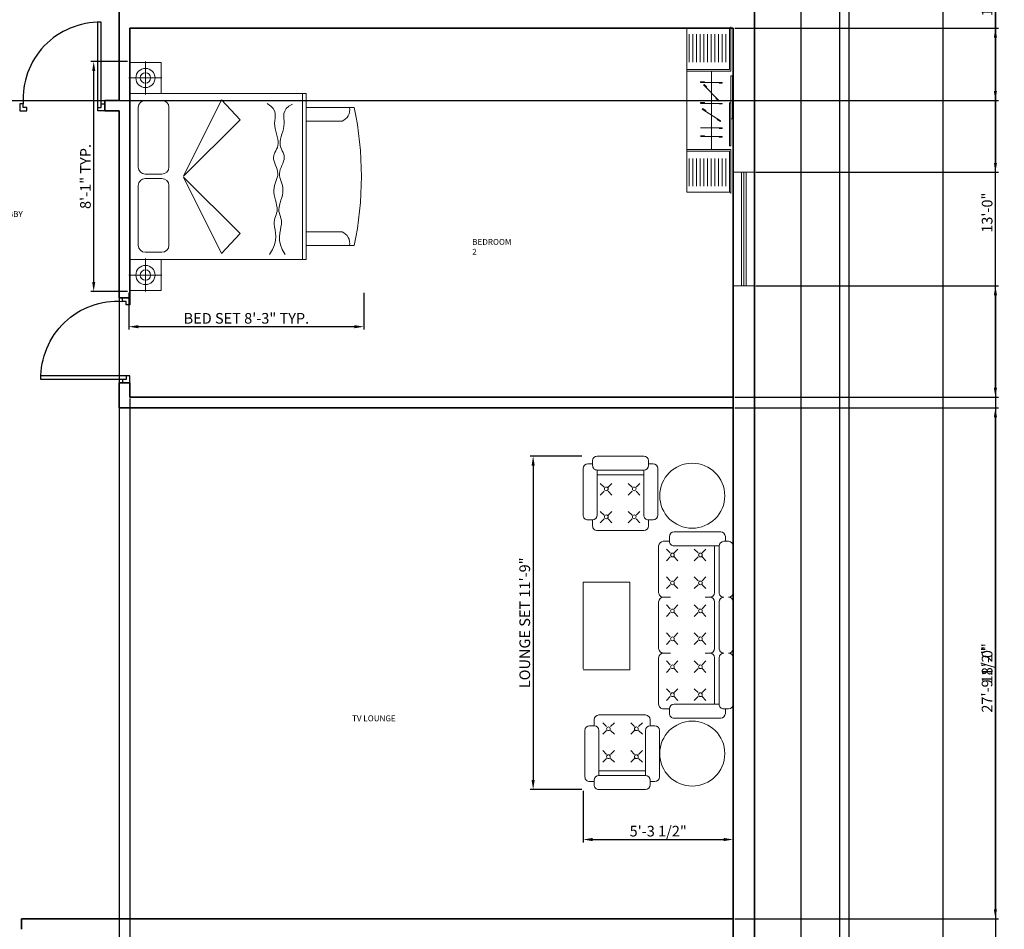
# Model space of a CAD drawing. Units: inches. Extents: x 1239 to 2276906, y 2273 to 321338.
# Tile 18 of 23: x 1620 to 2036, y 3026 to 3411. Entities that reach past the tile are written whole.
import ezdxf

# ---------------------------------------------------------------- set-up
doc = ezdxf.new("R2010")
doc.units = ezdxf.units.IN
for name, color, linetype, lineweight in [('A-ANNO-DIMS', 2, 'Continuous', 18), ('A-AREA-IDEN', 7, 'Continuous', 18), ('A-FLOR-CASE', 8, 'Continuous', 18), ('A-FURN', 8, 'Continuous', 13), ('C-PROP', 7, 'Continuous', 25), ('DOOR', 1, 'Continuous', 25), ('wall', 7, 'Continuous', 35), ('WINDOW', 50, 'Continuous', 18)]:
    doc.layers.add(name, color=color, linetype=linetype, lineweight=lineweight)
doc.styles.get("Standard").update_dxf_attribs({"font": 'arial.ttf'})
doc.dimstyles.new('ISO-25', dxfattribs={"dimtxt": 4.5, "dimasz": 4, "dimexe": 1.25, "dimexo": 0.625, "dimtad": 1, "dimdec": 1, "dimlunit": 3, "dimtxsty": 'Standard', "dimcen": 2.5, "dimadec": 0, "dimazin": 0, "dimtfac": 1, "dimtdec": 1, "dimtmove": 0, "dimatfit": 3, "dimfxl": 1, "dimarcsym": 0})

# ---------------------------------------------------------------- blocks, each defined once
blk = doc.blocks.new('A$C4F543DC7')
for p, q in [((0.013, 3.35, -0.169), (3.313, 3.35, -0.169)), ((0.463, 3.35, -0.169), (0.013, 3.35, -0.169)), ((0.013, 2.896, -0.169), (0.013, 3.35, -0.169)), ((0.013, 3.35, -0.169), (0.013, 2.896, -0.169)), ((0.238, 3.123, -0.439), (0.238, 3.361, -0.439)), ((0.463, 3.35, -0.169), (0.463, 0.8, -0.169)), ((2.863, 3.35, -0.169), (0.463, 3.35, -0.169)), ((0.463, 2.896, -0.169), (0.463, 3.35, -0.169)), ((2.863, 0.8, -0.169), (2.863, 3.35, -0.169)), ((2.863, 3.35, -0.169), (3.313, 3.35, -0.169)), ((2.863, 2.896, -0.169), (2.863, 3.35, -0.169)), ((3.089, 3.123, -0.439), (3.089, 3.361, -0.439)), ((3.313, 3.35, -0.169), (3.313, 2.896, -0.169)), ((3.313, 3.35, -0.169), (3.313, 2.896, -0.169)), ((1.535, 3.226, -0.169), (0.668, 3.226, -0.169)), ((2.664, 3.226, -0.169), (1.797, 3.226, -0.169)), ((0.238, 3.123, -0.439), (0, 3.123, -0.439)), ((0.238, 3.123, -0.439), (0.476, 3.123, -0.439)), ((0.238, 3.123, -0.439), (0.238, 2.885, -0.439)), ((0.568, 3.126, -0.169), (0.568, 2.884, -0.169)), ((1.635, 2.884, -0.169), (1.635, 3.126, -0.169)), ((1.697, 3.126, -0.169), (1.697, 2.884, -0.169)), ((2.764, 2.884, -0.169), (2.764, 3.126, -0.169)), ((3.089, 3.123, -0.439), (2.851, 3.123, -0.439)), ((3.089, 3.123, -0.439), (3.089, 2.885, -0.439)), ((3.089, 3.123, -0.439), (3.327, 3.123, -0.439)), ((0.463, 2.896, -0.169), (0.013, 2.896, -0.169)), ((0.013, 2.896, -0.169), (0.463, 2.896, -0.169)), ((0.463, 0.8, -0.169), (0.463, 2.896, -0.169)), ((2.863, 2.896, -0.169), (2.863, 0.8, -0.169)), ((3.313, 2.896, -0.169), (2.863, 2.896, -0.169)), ((3.313, 2.896, -0.169), (2.863, 2.896, -0.169)), ((0.668, 2.784, -0.169), (1.535, 2.784, -0.169)), ((1.797, 2.784, -0.169), (2.664, 2.784, -0.169)), ((1.653, 2.573, -0.169), (0.55, 2.025, -0.169)), ((0.841, 1.752, -0.169), (1.653, 2.573, -0.169)), ((2.481, 1.752, -0.169), (1.669, 2.573, -0.169)), ((1.669, 2.573, -0.169), (2.772, 2.025, -0.169)), ((0.55, 2.025, -0.169), (0.841, 1.752, -0.169)), ((2.772, 2.025, -0.169), (2.481, 1.752, -0.169)), ((0.537, 1.327, -0.169), (0.609, 1.284, -0.169)), ((0.609, 1.284, -0.169), (0.676, 1.257, -0.169)), ((2.648, 1.277, -0.169), (2.683, 1.312, -0.169)), ((2.683, 1.312, -0.169), (2.718, 1.364, -0.169)), ((0.533, 1.105, -0.169), (0.607, 1.146, -0.169)), ((0.607, 1.146, -0.169), (0.674, 1.171, -0.169)), ((0.674, 1.171, -0.169), (0.736, 1.183, -0.169)), ((0.676, 1.257, -0.169), (0.737, 1.243, -0.169)), ((0.736, 1.183, -0.169), (0.793, 1.185, -0.169)), ((0.737, 1.243, -0.169), (0.794, 1.239, -0.169)), ((0.793, 1.185, -0.169), (0.845, 1.18, -0.169)), ((0.794, 1.239, -0.169), (0.846, 1.242, -0.169)), ((0.845, 1.18, -0.169), (0.891, 1.172, -0.169)), ((0.846, 1.242, -0.169), (0.893, 1.249, -0.169)), ((0.891, 1.172, -0.169), (0.933, 1.163, -0.169)), ((0.893, 1.249, -0.169), (0.935, 1.256, -0.169)), ((0.933, 1.163, -0.169), (0.97, 1.156, -0.169)), ((0.935, 1.256, -0.169), (0.972, 1.261, -0.169)), ((0.97, 1.156, -0.169), (1.003, 1.155, -0.169)), ((0.972, 1.261, -0.169), (1.004, 1.262, -0.169)), ((1.003, 1.155, -0.169), (1.032, 1.158, -0.169)), ((1.004, 1.262, -0.169), (1.033, 1.258, -0.169)), ((1.032, 1.158, -0.169), (1.058, 1.164, -0.169)), ((1.033, 1.258, -0.169), (1.06, 1.251, -0.169)), ((1.058, 1.164, -0.169), (1.083, 1.172, -0.169)), ((1.06, 1.251, -0.169), (1.084, 1.242, -0.169)), ((1.083, 1.172, -0.169), (1.107, 1.18, -0.169)), ((1.084, 1.242, -0.169), (1.108, 1.234, -0.169)), ((1.107, 1.18, -0.169), (1.132, 1.187, -0.169)), ((1.108, 1.234, -0.169), (1.132, 1.226, -0.169)), ((1.132, 1.226, -0.169), (1.158, 1.22, -0.169)), ((1.132, 1.187, -0.169), (1.157, 1.192, -0.169)), ((1.157, 1.192, -0.169), (1.185, 1.193, -0.169)), ((1.158, 1.22, -0.169), (1.185, 1.218, -0.169)), ((1.185, 1.218, -0.169), (1.216, 1.22, -0.169)), ((1.185, 1.193, -0.169), (1.216, 1.19, -0.169)), ((1.216, 1.22, -0.169), (1.25, 1.226, -0.169)), ((1.216, 1.19, -0.169), (1.249, 1.183, -0.169)), ((1.249, 1.183, -0.169), (1.284, 1.173, -0.169)), ((1.25, 1.226, -0.169), (1.285, 1.235, -0.169)), ((1.284, 1.173, -0.169), (1.321, 1.163, -0.169)), ((1.285, 1.235, -0.169), (1.322, 1.244, -0.169)), ((1.321, 1.163, -0.169), (1.358, 1.152, -0.169)), ((1.322, 1.244, -0.169), (1.359, 1.253, -0.169)), ((1.358, 1.152, -0.169), (1.394, 1.143, -0.169)), ((1.359, 1.253, -0.169), (1.396, 1.261, -0.169)), ((1.394, 1.143, -0.169), (1.431, 1.137, -0.169)), ((1.396, 1.261, -0.169), (1.433, 1.266, -0.169)), ((1.433, 1.266, -0.169), (1.468, 1.268, -0.169)), ((1.468, 1.268, -0.169), (1.501, 1.264, -0.169)), ((1.499, 1.137, -0.169), (1.531, 1.143, -0.169)), ((1.501, 1.264, -0.169), (1.532, 1.257, -0.169)), ((1.531, 1.143, -0.169), (1.561, 1.152, -0.169)), ((1.532, 1.257, -0.169), (1.562, 1.247, -0.169)), ((1.561, 1.152, -0.169), (1.59, 1.162, -0.169)), ((1.562, 1.247, -0.169), (1.591, 1.237, -0.169)), ((1.59, 1.162, -0.169), (1.619, 1.172, -0.169)), ((1.591, 1.237, -0.169), (1.62, 1.226, -0.169)), ((1.619, 1.172, -0.169), (1.648, 1.18, -0.169)), ((1.62, 1.226, -0.169), (1.648, 1.217, -0.169)), ((1.648, 1.217, -0.169), (1.676, 1.211, -0.169)), ((1.648, 1.18, -0.169), (1.676, 1.185, -0.169)), ((1.676, 1.211, -0.169), (1.705, 1.209, -0.169)), ((1.676, 1.185, -0.169), (1.705, 1.186, -0.169)), ((1.705, 1.209, -0.169), (1.735, 1.212, -0.169)), ((1.705, 1.186, -0.169), (1.734, 1.182, -0.169)), ((1.734, 1.182, -0.169), (1.764, 1.173, -0.169)), ((1.735, 1.212, -0.169), (1.765, 1.22, -0.169)), ((1.764, 1.173, -0.169), (1.794, 1.162, -0.169)), ((1.765, 1.22, -0.169), (1.795, 1.23, -0.169)), ((1.794, 1.162, -0.169), (1.824, 1.149, -0.169)), ((1.795, 1.23, -0.169), (1.826, 1.242, -0.169)), ((1.824, 1.149, -0.169), (1.854, 1.137, -0.169)), ((1.826, 1.242, -0.169), (1.856, 1.253, -0.169)), ((1.856, 1.253, -0.169), (1.885, 1.263, -0.169)), ((1.885, 1.263, -0.169), (1.913, 1.27, -0.169)), ((1.913, 1.27, -0.169), (1.94, 1.272, -0.169)), ((1.94, 1.272, -0.169), (1.965, 1.269, -0.169)), ((1.965, 1.269, -0.169), (1.989, 1.262, -0.169)), ((1.989, 1.262, -0.169), (2.012, 1.251, -0.169)), ((2.011, 1.134, -0.169), (2.034, 1.145, -0.169)), ((2.012, 1.251, -0.169), (2.036, 1.239, -0.169)), ((2.034, 1.145, -0.169), (2.059, 1.157, -0.169)), ((2.036, 1.239, -0.169), (2.06, 1.227, -0.169)), ((2.059, 1.157, -0.169), (2.084, 1.167, -0.169)), ((2.06, 1.227, -0.169), (2.085, 1.216, -0.169)), ((2.084, 1.167, -0.169), (2.111, 1.174, -0.169)), ((2.085, 1.216, -0.169), (2.112, 1.208, -0.169)), ((2.111, 1.174, -0.169), (2.14, 1.177, -0.169)), ((2.112, 1.208, -0.169), (2.141, 1.204, -0.169)), ((2.14, 1.177, -0.169), (2.172, 1.175, -0.169)), ((2.141, 1.204, -0.169), (2.172, 1.205, -0.169)), ((2.172, 1.205, -0.169), (2.206, 1.21, -0.169)), ((2.172, 1.175, -0.169), (2.206, 1.169, -0.169)), ((2.206, 1.21, -0.169), (2.242, 1.218, -0.169)), ((2.206, 1.169, -0.169), (2.241, 1.16, -0.169)), ((2.241, 1.16, -0.169), (2.278, 1.149, -0.169)), ((2.242, 1.218, -0.169), (2.279, 1.228, -0.169)), ((2.278, 1.149, -0.169), (2.316, 1.138, -0.169)), ((2.279, 1.228, -0.169), (2.317, 1.238, -0.169)), ((2.317, 1.238, -0.169), (2.356, 1.246, -0.169)), ((2.356, 1.246, -0.169), (2.394, 1.253, -0.169)), ((2.394, 1.253, -0.169), (2.433, 1.255, -0.169)), ((2.433, 1.255, -0.169), (2.47, 1.253, -0.169)), ((2.47, 1.253, -0.169), (2.506, 1.249, -0.169)), ((2.506, 1.249, -0.169), (2.542, 1.246, -0.169)), ((2.542, 1.246, -0.169), (2.578, 1.248, -0.169)), ((2.578, 1.248, -0.169), (2.613, 1.257, -0.169)), ((2.613, 1.257, -0.169), (2.648, 1.277, -0.169)), ((1.431, 1.137, -0.169), (1.466, 1.135, -0.169)), ((1.466, 1.135, -0.169), (1.499, 1.137, -0.169)), ((1.854, 1.137, -0.169), (1.883, 1.126, -0.169)), ((1.883, 1.126, -0.169), (1.911, 1.119, -0.169)), ((1.911, 1.119, -0.169), (1.937, 1.115, -0.169)), ((1.937, 1.115, -0.169), (1.963, 1.118, -0.169)), ((1.963, 1.118, -0.169), (1.987, 1.124, -0.169)), ((1.987, 1.124, -0.169), (2.011, 1.134, -0.169)), ((2.316, 1.138, -0.169), (2.354, 1.128, -0.169)), ((2.354, 1.128, -0.169), (2.392, 1.121, -0.169)), ((2.392, 1.121, -0.169), (2.43, 1.117, -0.169)), ((2.43, 1.117, -0.169), (2.468, 1.118, -0.169)), ((2.468, 1.118, -0.169), (2.504, 1.121, -0.169)), ((2.504, 1.121, -0.169), (2.54, 1.123, -0.169)), ((2.54, 1.123, -0.169), (2.576, 1.12, -0.169)), ((2.576, 1.12, -0.169), (2.611, 1.109, -0.169)), ((2.611, 1.109, -0.169), (2.645, 1.088, -0.169)), ((2.645, 1.088, -0.169), (2.679, 1.052, -0.169)), ((2.679, 1.052, -0.169), (2.712, 0.999, -0.169)), ((0.463, 0.85, -0.169), (2.863, 0.85, -0.169)), ((0.463, 0.8, -0.169), (2.863, 0.8, -0.169)), ((0.663, 0.8, -0.169), (0.463, 0.8, -0.169)), ((0.663, 0.8, -0.169), (2.663, 0.8, -0.169)), ((0.663, 0.104, -0.169), (0.663, 0.8, -0.169)), ((0.663, 0.104, -0.169), (0.663, 0.8, -0.169)), ((0.863, 0.281, -0.169), (0.863, 0.8, -0.169)), ((2.463, 0.8, -0.169), (2.463, 0.281, -0.169)), ((2.863, 0.8, -0.169), (2.663, 0.8, -0.169)), ((2.663, 0.8, -0.169), (2.663, 0.104, -0.169)), ((2.663, 0.8, -0.169), (2.663, 0.104, -0.169))]:
    blk.add_line(p, q)
for centre, radius in [((0.238, 3.123, -0.439), 0.139), ((0.238, 3.123, -0.439), 0.075), ((3.089, 3.123, -0.439), 0.139), ((3.089, 3.123, -0.439), 0.075)]:
    blk.add_circle(centre, radius)
for centre, radius, start, end in [((0.668, 3.126, -0.169), 0.1, 90, 180), ((1.535, 3.126, -0.169), 0.1, 0, 90), ((1.797, 3.126, -0.169), 0.1, 90, 180), ((2.664, 3.126, -0.169), 0.1, 0, 90), ((0.668, 2.884, -0.169), 0.1, 180, 270), ((1.535, 2.884, -0.169), 0.1, 270, 0), ((1.797, 2.884, -0.169), 0.1, 180, 270), ((2.664, 2.884, -0.169), 0.1, 270, 0), ((0.699, 0.347, -0.169), 0.177, 258.2616, 338.032), ((2.627, 0.347, -0.169), 0.177, 201.968, 281.7384), ((1.663, 4.86, -0.169), 4.86, 258.1252, 281.8748), ((1.663, 4.86, -0.169), 4.86, 258.1252, 281.8748)]:
    blk.add_arc(centre, radius, start, end)
blk = doc.blocks.new('A$C34930FF8')
at = {"ltscale": 0.05}
for p, q in [((0, 2252), (0, 17)), ((600, 2252), (0, 2252)), ((185, 1513), (185, 1521)), ((227, 1479), (233, 1485)), ((238, 1513), (238, 1521)), ((437, 1513), (437, 1504)), ((482, 1513), (482, 1504)), ((264, 1442), (270, 1448)), ((185, 1229), (185, 1238)), ((238, 1229), (238, 1238)), ((398, 1304), (392, 1298)), ((435, 1266), (429, 1260)), ((437, 1228), (437, 1220)), ((482, 1228), (482, 1220)), ((209, 1150), (214, 1157)), ((253, 1122), (258, 1129)), ((415, 1018), (411, 1010)), ((459, 989), (455, 982)), ((482, 895), (482, 886)), ((238, 775), (238, 784)), ((437, 775), (437, 767)), ((482, 775), (482, 767)), ((600, 17), (0, 17))]:
    blk.add_line(p, q, dxfattribs=at)
for p, q in [((30, 1791), (30, 2169)), ((80, 1791), (80, 2169)), ((130, 1791), (130, 2169)), ((180, 1791), (180, 2169)), ((230, 1791), (230, 2169)), ((280, 1791), (280, 2169)), ((330, 1791), (330, 2169)), ((380, 1791), (380, 2169)), ((430, 1791), (430, 2169)), ((480, 1791), (480, 2169)), ((530, 1791), (530, 2169)), ((580, 1691), (580, 2252)), ((600, 1669), (600, 2269)), ((580, 1691), (0, 1691)), ((600, 1669), (0, 1669)), ((335, 1666), (335, 603)), ((238, 1521), (185, 1521)), ((482, 1513), (185, 1513)), ((435, 1266), (227, 1479)), ((270, 1448), (233, 1485)), ((437, 1504), (482, 1504)), ((600, 1603), (620, 1603)), ((600, 1019), (600, 1603)), ((620, 1603), (620, 1019)), ((238, 1238), (185, 1238)), ((482, 1228), (185, 1228)), ((429, 1260), (392, 1298)), ((437, 1220), (482, 1220)), ((600, 1233), (580, 1233)), ((580, 1233), (580, 649)), ((600, 649), (600, 1233)), ((459, 989), (209, 1150)), ((258, 1129), (214, 1157)), ((455, 982), (411, 1010)), ((620, 1019), (600, 1019)), ((482, 895), (185, 895)), ((437, 886), (482, 886)), ((238, 784), (185, 784)), ((482, 775), (185, 775)), ((437, 767), (482, 767)), ((600, 600), (0, 600)), ((580, 578), (0, 578)), ((580, 649), (600, 649)), ((580, 578), (580, 17)), ((600, 600), (600, 0)), ((30, 478), (30, 100)), ((80, 478), (80, 100)), ((130, 478), (130, 100)), ((180, 478), (180, 100)), ((230, 478), (230, 100)), ((280, 478), (280, 100)), ((330, 478), (330, 100)), ((380, 478), (380, 100)), ((430, 478), (430, 100)), ((480, 478), (480, 100)), ((530, 478), (530, 100))]:
    blk.add_line(p, q)
blk = doc.blocks.new('A$C144B2C1F')
at = {"linetype": 'ByBlock'}
for p, q in [((1465, 1610), (965, 1610)), ((2065, 1610), (1565, 1610)), ((2665, 1610), (2165, 1610)), ((914, 1526), (864, 1526)), ((915, 1560), (915, 1510)), ((2764, 1526), (2714, 1526)), ((2715, 1510), (2715, 1560)), ((814, 1476), (814, 976)), ((964, 976), (964, 1460)), ((965, 1460), (1465, 1460)), ((965, 1410), (1465, 1410)), ((1565, 1460), (2065, 1460)), ((1565, 1410), (2065, 1410)), ((2165, 1460), (2665, 1460)), ((2165, 1410), (2664, 1410)), ((2664, 1460), (2664, 976)), ((2814, 976), (2814, 1476)), ((1040, 1277), (998, 1317)), ((1081, 1277), (1123, 1317)), ((1340, 1277), (1298, 1317)), ((1381, 1277), (1423, 1317)), ((1515, 1311), (1515, 1360)), ((1640, 1277), (1598, 1317)), ((1681, 1277), (1723, 1317)), ((1940, 1277), (1898, 1317)), ((1981, 1277), (2023, 1317)), ((2115, 1311), (2115, 1360)), ((2240, 1277), (2198, 1317)), ((2281, 1277), (2323, 1317)), ((2540, 1277), (2498, 1317)), ((2581, 1277), (2623, 1317)), ((1040, 1235), (998, 1193)), ((1081, 1235), (1123, 1193)), ((1340, 1235), (1298, 1193)), ((1381, 1235), (1423, 1193)), ((1640, 1235), (1598, 1193)), ((1681, 1235), (1723, 1193)), ((1940, 1235), (1898, 1193)), ((1981, 1235), (2023, 1193)), ((2240, 1235), (2198, 1193)), ((2281, 1235), (2323, 1193)), ((2540, 1235), (2498, 1193)), ((2581, 1235), (2623, 1193)), ((1040, 977), (998, 1017)), ((1081, 977), (1123, 1017)), ((1340, 977), (1298, 1017)), ((1381, 977), (1423, 1017)), ((1640, 977), (1598, 1017)), ((1681, 977), (1723, 1017)), ((1940, 977), (1898, 1017)), ((1981, 977), (2023, 1017)), ((2240, 977), (2198, 1017)), ((2281, 977), (2323, 1017)), ((2540, 977), (2498, 1017)), ((2581, 977), (2623, 1017)), ((864, 926), (914, 926)), ((915, 926), (915, 860)), ((1040, 935), (998, 893)), ((1081, 935), (1123, 893)), ((1340, 935), (1298, 893)), ((1381, 935), (1423, 893)), ((1515, 860), (1515, 937)), ((1515, 926), (1515, 860)), ((1640, 935), (1598, 893)), ((1681, 935), (1723, 893)), ((1940, 935), (1898, 893)), ((1981, 935), (2023, 893)), ((2115, 860), (2115, 937)), ((2115, 926), (2115, 860)), ((2240, 935), (2198, 893)), ((2281, 935), (2323, 893)), ((2540, 935), (2498, 893)), ((2581, 935), (2623, 893)), ((2714, 926), (2764, 926)), ((2715, 860), (2715, 926)), ((84, 750), (84, 700)), ((634, 800), (134, 800)), ((684, 700), (684, 750)), ((1129, 810), (965, 810)), ((1465, 810), (1088, 810)), ((1729, 810), (1565, 810)), ((2065, 810), (1688, 810)), ((2329, 810), (2165, 810)), ((2665, 810), (2288, 810)), ((2896, 769), (2896, 719)), ((3446, 819), (2946, 819)), ((3496, 719), (3496, 769)), ((0, 651), (0, 151)), ((100, 701), (50, 701)), ((150, 151), (150, 651)), ((150, 650), (634, 650)), ((200, 151), (200, 650)), ((750, 701), (684, 701)), ((800, 651), (800, 274)), ((2780, 504), (2780, 668)), ((2896, 718), (2830, 718)), ((2905, 593), (2863, 635)), ((2946, 669), (3430, 669)), ((2948, 593), (2987, 635)), ((3205, 593), (3163, 635)), ((3248, 593), (3287, 635)), ((3380, 668), (3380, 169)), ((3430, 668), (3430, 168)), ((3530, 718), (3480, 718)), ((3580, 168), (3580, 668)), ((333, 567), (293, 608)), ((375, 567), (418, 608)), ((633, 567), (593, 608)), ((675, 567), (718, 608)), ((2780, 168), (2780, 545)), ((2905, 552), (2863, 510)), ((2948, 552), (2987, 510)), ((3205, 552), (3163, 510)), ((3248, 552), (3287, 510)), ((333, 525), (293, 484)), ((375, 525), (418, 484)), ((633, 525), (593, 484)), ((675, 525), (718, 484)), ((2295, 501), (1355, 501)), ((1355, 501), (1355, 1)), ((2295, 1), (2295, 501)), ((2905, 293), (2863, 335)), ((2948, 293), (2987, 335)), ((3205, 293), (3163, 335)), ((3248, 293), (3287, 335)), ((333, 267), (293, 308)), ((333, 225), (293, 184)), ((375, 267), (418, 308)), ((375, 225), (418, 184)), ((633, 267), (593, 308)), ((633, 225), (593, 184)), ((675, 267), (718, 308)), ((675, 225), (718, 184)), ((800, 314), (800, 151)), ((2905, 252), (2863, 210)), ((2948, 252), (2987, 210)), ((3205, 252), (3163, 210)), ((3248, 252), (3287, 210)), ((634, 150), (150, 150)), ((2830, 118), (2896, 118)), ((2896, 119), (2896, 69)), ((3430, 169), (2946, 169)), ((3480, 118), (3530, 118)), ((3496, 69), (3496, 119)), ((50, 101), (100, 101)), ((84, 100), (84, 50)), ((134, 0), (634, 0)), ((684, 101), (750, 101)), ((684, 50), (684, 100)), ((1355, 1), (2285, 1)), ((2946, 19), (3446, 19))]:
    blk.add_line(p, q, dxfattribs=at)
for centre, radius in [((425, 1171), 349), ((3195, 1171), 349), ((1062, 1258), 20), ((1362, 1258), 20), ((1662, 1258), 20), ((1962, 1258), 20), ((2262, 1258), 20), ((2562, 1258), 20), ((1062, 958), 20), ((1362, 958), 20), ((1662, 958), 20), ((1962, 958), 20), ((2262, 958), 20), ((2562, 958), 20), ((352, 548), 20), ((652, 548), 20), ((2928, 571), 20), ((3228, 571), 20), ((352, 248), 20), ((652, 248), 20), ((2928, 271), 20), ((3228, 271), 20)]:
    blk.add_circle(centre, radius, dxfattribs=at)
for centre, start, end in [((965, 1560), 90, 180), ((965, 1560), 90, 180), ((1465, 1560), 0, 90), ((1565, 1560), 90, 180), ((1565, 1560), 90, 180), ((2065, 1560), 0, 90), ((2165, 1560), 90, 180), ((2165, 1560), 90, 180), ((2665, 1560), 0, 90), ((864, 1476), 90, 180), ((965, 1510), 180, 270), ((1465, 1510), 270, 0), ((1565, 1510), 180, 270), ((2065, 1510), 270, 0), ((2165, 1510), 180, 270), ((2665, 1510), 270, 0), ((2764, 1476), 0, 90), ((1465, 1360), 0, 90), ((1565, 1360), 90, 180), ((2065, 1360), 0, 90), ((2165, 1360), 90, 180), ((864, 976), 180, 270), ((914, 976), 270, 0), ((2714, 976), 180, 270), ((2764, 976), 270, 0), ((965, 860), 180, 270), ((1465, 860), 270, 0), ((1565, 860), 180, 270), ((2065, 860), 270, 0), ((2165, 860), 180, 270), ((2665, 860), 270, 0), ((134, 750), 90, 180), ((634, 750), 0, 90), ((2946, 769), 90, 180), ((3446, 769), 0, 90), ((50, 651), 90, 180), ((100, 651), 0, 90), ((634, 700), 270, 0), ((750, 651), 0, 90), ((2830, 668), 90, 180), ((2946, 719), 180, 270), ((3480, 668), 90, 180), ((3530, 668), 0, 90), ((3530, 668), 0, 90), ((50, 151), 180, 270), ((50, 151), 180, 270), ((100, 151), 270, 0), ((634, 100), 0, 90), ((750, 151), 270, 0), ((2830, 168), 180, 270), ((2946, 119), 90, 180), ((3480, 168), 180, 270), ((3530, 168), 270, 0), ((134, 50), 180, 270), ((634, 50), 270, 0), ((2946, 69), 180, 270), ((3446, 69), 270, 0)]:
    blk.add_arc(centre, 50, start, end, dxfattribs=at)
blk = doc.blocks.new('*D38')
at = {"layer": 'A-ANNO-DIMS', "color": 0, "lineweight": -2, "transparency": 16777216}
for p, q in [((1971.01, 3545.9), (2011.25, 3545.9)), ((2010, 3541.9), (2010, 2342.75)), ((1971.01, 2338.75), (2011.25, 2338.75))]:
    blk.add_line(p, q, dxfattribs=at)
at = {"layer": 'A-ANNO-DIMS', "color": 0, "transparency": 16777216}
for points in [[(2009.33, 3541.9), (2010.67, 3541.9), (2010, 3545.9)], [(2009.33, 2342.75), (2010.67, 2342.75), (2010, 2338.75)]]:
    blk.add_solid(points, dxfattribs=at)
at = {"layer": 'Defpoints', "color": 0, "transparency": 16777216}
for p in [(1970.38, 3545.9), (1970.38, 2338.75), (2010, 2338.75)]:
    blk.add_point(p, dxfattribs=at)
at = {"layer": 'A-ANNO-DIMS', "color": 0, "transparency": 16777216, "insert": (2007.08, 2942.32), "char_height": 4.5, "attachment_point": 5, "rotation": 90}
blk.add_mtext('100\'-7.2"', dxfattribs=at)
blk = doc.blocks.new('*D40')
at = {"layer": 'A-ANNO-DIMS', "color": 0, "lineweight": -2, "transparency": 16777216}
for p, q in [((1931.01, 3505.9), (1951.25, 3505.9)), ((1950, 3501.9), (1950, 2354)), ((1931.01, 2350), (1951.25, 2350))]:
    blk.add_line(p, q, dxfattribs=at)
at = {"layer": 'A-ANNO-DIMS', "color": 0, "transparency": 16777216}
for points in [[(1949.33, 3501.9), (1950.67, 3501.9), (1950, 3505.9)], [(1949.33, 2354), (1950.67, 2354), (1950, 2350)]]:
    blk.add_solid(points, dxfattribs=at)
at = {"layer": 'Defpoints', "color": 0, "transparency": 16777216}
for p in [(1930.38, 3505.9), (1930.38, 2350), (1950, 2350)]:
    blk.add_point(p, dxfattribs=at)
at = {"layer": 'A-ANNO-DIMS', "color": 0, "transparency": 16777216, "insert": (1947.08, 2927.95), "char_height": 4.5, "attachment_point": 5, "rotation": 90}
blk.add_mtext('96\'-3.9"', dxfattribs=at)
blk = doc.blocks.new('DOOR-SINGLE-36')
for p, q in [((33, 1.5), (33, 37.5)), ((34.5, 1.5), (34.5, 37.5)), ((0, 3), (0, 0)), ((1.5, 3), (0, 3)), ((0, 0), (3, 0)), ((1.5, 1.5), (1.5, 3)), ((3, 1.5), (1.5, 1.5)), ((3, 0), (3, 1.5)), ((33, 0), (33, 1.5)), ((33, 1.5), (34.5, 1.5)), ((36, 0), (33, 0)), ((34.5, 1.5), (34.5, 3)), ((34.5, 3), (36, 3)), ((36, 3), (36, 0))]:
    blk.add_line(p, q)
blk.add_arc((33.75, 5.18), 32.32, 88.6705, 183.8756)
blk = doc.blocks.new('WIN-48')
for p, q in [((0, 48), (9, 48)), ((0, 0), (0, 48)), ((3.5, 0), (3.5, 48)), ((4.5, 0), (4.5, 48)), ((5.5, 0), (5.5, 48)), ((9, 0), (9, 48)), ((0, 0), (9, 0))]:
    blk.add_line(p, q)
blk = doc.blocks.new('*D64')
at = {"layer": 'A-ANNO-DIMS', "color": 0, "lineweight": -2, "transparency": 16777216}
for p, q in [((1857.36, 3226.47), (1835.59, 3226.47)), ((1836.84, 3222.47), (1836.84, 3089.51)), ((1857.36, 3085.51), (1835.59, 3085.51))]:
    blk.add_line(p, q, dxfattribs=at)
at = {"layer": 'A-ANNO-DIMS', "color": 0, "transparency": 16777216}
for points in [[(1836.18, 3222.47), (1837.51, 3222.47), (1836.84, 3226.47)], [(1836.18, 3089.51), (1837.51, 3089.51), (1836.84, 3085.51)]]:
    blk.add_solid(points, dxfattribs=at)
at = {"layer": 'Defpoints', "color": 0, "transparency": 16777216}
for p in [(1857.99, 3226.47), (1836.84, 3085.51), (1857.99, 3085.51)]:
    blk.add_point(p, dxfattribs=at)
at = {"layer": 'A-ANNO-DIMS', "color": 0, "transparency": 16777216, "insert": (1833.89, 3155.99), "char_height": 4.5, "attachment_point": 5, "rotation": 90}
blk.add_mtext('LOUNGE SET 11\'-9"', dxfattribs=at)
blk = doc.blocks.new('*D65')
at = {"layer": 'A-ANNO-DIMS', "color": 0, "lineweight": -2, "transparency": 16777216}
for p, q in [((1857.99, 3084.89), (1857.99, 3063.12)), ((1921.38, 3084.89), (1921.38, 3063.12)), ((1861.99, 3064.37), (1917.38, 3064.37))]:
    blk.add_line(p, q, dxfattribs=at)
at = {"layer": 'A-ANNO-DIMS', "color": 0, "transparency": 16777216}
for points in [[(1861.99, 3065.03), (1861.99, 3063.7), (1857.99, 3064.37)], [(1917.38, 3065.03), (1917.38, 3063.7), (1921.38, 3064.37)]]:
    blk.add_solid(points, dxfattribs=at)
at = {"layer": 'Defpoints', "color": 0, "transparency": 16777216}
for p in [(1857.99, 3085.51), (1921.38, 3085.51), (1921.38, 3064.37)]:
    blk.add_point(p, dxfattribs=at)
at = {"layer": 'A-ANNO-DIMS', "color": 0, "transparency": 16777216, "insert": (1889.69, 3067.32), "char_height": 4.5, "attachment_point": 5}
blk.add_mtext('5\'-3 1/2"', dxfattribs=at)
blk = doc.blocks.new('*D68')
at = {"layer": 'A-ANNO-DIMS', "color": 0, "lineweight": -2, "transparency": 16777216}
for p, q in [((1666.05, 3295.46), (1666.05, 3279.94)), ((1765.3, 3295.46), (1765.3, 3279.94)), ((1761.3, 3281.19), (1670.05, 3281.19))]:
    blk.add_line(p, q, dxfattribs=at)
at = {"layer": 'A-ANNO-DIMS', "color": 0, "transparency": 16777216}
for points in [[(1670.05, 3281.86), (1670.05, 3280.53), (1666.05, 3281.19)], [(1761.3, 3281.86), (1761.3, 3280.53), (1765.3, 3281.19)]]:
    blk.add_solid(points, dxfattribs=at)
at = {"layer": 'Defpoints', "color": 0, "transparency": 16777216}
for p in [(1666.05, 3296.08), (1765.3, 3296.08), (1666.05, 3281.19)]:
    blk.add_point(p, dxfattribs=at)
at = {"layer": 'A-ANNO-DIMS', "color": 0, "transparency": 16777216, "insert": (1715.68, 3284.15), "char_height": 4.5, "attachment_point": 5}
blk.add_mtext('BED SET 8\'-3" TYP.', dxfattribs=at)
blk = doc.blocks.new('*D69')
at = {"layer": 'A-ANNO-DIMS', "color": 0, "lineweight": -2, "transparency": 16777216}
for p, q in [((1665.43, 3393.31), (1649.91, 3393.31)), ((1651.16, 3300.08), (1651.16, 3389.31)), ((1665.43, 3296.08), (1649.91, 3296.08))]:
    blk.add_line(p, q, dxfattribs=at)
at = {"layer": 'A-ANNO-DIMS', "color": 0, "transparency": 16777216}
for points in [[(1650.5, 3389.31), (1651.83, 3389.31), (1651.16, 3393.31)], [(1650.5, 3300.08), (1651.83, 3300.08), (1651.16, 3296.08)]]:
    blk.add_solid(points, dxfattribs=at)
at = {"layer": 'Defpoints', "color": 0, "transparency": 16777216}
for p in [(1651.16, 3393.31), (1666.05, 3393.31), (1666.05, 3296.08)]:
    blk.add_point(p, dxfattribs=at)
at = {"layer": 'A-ANNO-DIMS', "color": 0, "transparency": 16777216, "insert": (1648.24, 3344.7), "char_height": 4.5, "attachment_point": 5, "rotation": 90}
blk.add_mtext('8\'-1" TYP.', dxfattribs=at)
blk = doc.blocks.new('*D85')
at = {"layer": 'A-ANNO-DIMS', "color": 0, "lineweight": -2, "transparency": 16777216}
for p, q in [((1470.51, 3496.9), (2033.43, 3496.9)), ((2032.18, 3380.9), (2032.18, 3492.9)), ((1470.51, 3376.9), (2033.43, 3376.9))]:
    blk.add_line(p, q, dxfattribs=at)
at = {"layer": 'A-ANNO-DIMS', "color": 0, "transparency": 16777216}
for points in [[(2031.52, 3492.9), (2032.85, 3492.9), (2032.18, 3496.9)], [(2031.52, 3380.9), (2032.85, 3380.9), (2032.18, 3376.9)]]:
    blk.add_solid(points, dxfattribs=at)
at = {"layer": 'Defpoints', "color": 0, "transparency": 16777216}
for p in [(1469.88, 3496.9), (2032.18, 3496.9), (1469.88, 3376.9)]:
    blk.add_point(p, dxfattribs=at)
at = {"layer": 'A-ANNO-DIMS', "color": 0, "transparency": 16777216, "insert": (2029.26, 3436.9), "char_height": 4.5, "attachment_point": 5, "rotation": 90}
blk.add_mtext('10\'-0"', dxfattribs=at)
blk = doc.blocks.new('*D87')
at = {"layer": 'A-ANNO-DIMS', "color": 0, "lineweight": -2, "transparency": 16777216}
for p, q in [((1666.38, 3250.77), (1666.38, 2275.7)), ((1921.38, 3250.77), (1921.38, 2275.7)), ((1670.38, 2276.95), (1917.38, 2276.95))]:
    blk.add_line(p, q, dxfattribs=at)
at = {"layer": 'A-ANNO-DIMS', "color": 0, "transparency": 16777216}
for points in [[(1670.38, 2277.61), (1670.38, 2276.28), (1666.38, 2276.95)], [(1917.38, 2277.61), (1917.38, 2276.28), (1921.38, 2276.95)]]:
    blk.add_solid(points, dxfattribs=at)
at = {"layer": 'Defpoints', "color": 0, "transparency": 16777216}
for p in [(1666.38, 3251.4), (1921.38, 3251.4), (1921.38, 2276.95)]:
    blk.add_point(p, dxfattribs=at)
at = {"layer": 'A-ANNO-DIMS', "color": 0, "transparency": 16777216, "insert": (1793.88, 2279.87), "char_height": 4.5, "attachment_point": 5}
blk.add_mtext('21\'-3"', dxfattribs=at)
blk = doc.blocks.new('*D88')
at = {"layer": 'A-ANNO-DIMS', "color": 0, "lineweight": -2, "transparency": 16777216}
for p, q in [((1922.01, 3407.4), (2033.43, 3407.4)), ((2032.18, 3255.4), (2032.18, 3403.4)), ((1922.01, 3251.4), (2033.43, 3251.4))]:
    blk.add_line(p, q, dxfattribs=at)
at = {"layer": 'A-ANNO-DIMS', "color": 0, "transparency": 16777216}
for points in [[(2031.52, 3403.4), (2032.85, 3403.4), (2032.18, 3407.4)], [(2031.52, 3255.4), (2032.85, 3255.4), (2032.18, 3251.4)]]:
    blk.add_solid(points, dxfattribs=at)
at = {"layer": 'Defpoints', "color": 0, "transparency": 16777216}
for p in [(1921.38, 3407.4), (2032.18, 3407.4), (1921.38, 3251.4)]:
    blk.add_point(p, dxfattribs=at)
at = {"layer": 'A-ANNO-DIMS', "color": 0, "transparency": 16777216, "insert": (2029.26, 3329.4), "char_height": 4.5, "attachment_point": 5, "rotation": 90}
blk.add_mtext('13\'-0"', dxfattribs=at)
blk = doc.blocks.new('*D94')
at = {"layer": 'A-ANNO-DIMS', "color": 0, "lineweight": -2, "transparency": 16777216}
for p, q in [((1922.01, 3246.9), (2033.43, 3246.9)), ((2032.18, 3034.9), (2032.18, 3242.9)), ((1922.01, 3030.9), (2033.43, 3030.9))]:
    blk.add_line(p, q, dxfattribs=at)
at = {"layer": 'A-ANNO-DIMS', "color": 0, "transparency": 16777216}
for points in [[(2031.52, 3242.9), (2032.85, 3242.9), (2032.18, 3246.9)], [(2031.52, 3034.9), (2032.85, 3034.9), (2032.18, 3030.9)]]:
    blk.add_solid(points, dxfattribs=at)
at = {"layer": 'Defpoints', "color": 0, "transparency": 16777216}
for p in [(1921.38, 3246.9), (2032.18, 3246.9), (1921.38, 3030.9)]:
    blk.add_point(p, dxfattribs=at)
at = {"layer": 'A-ANNO-DIMS', "color": 0, "transparency": 16777216, "insert": (2029.26, 3138.9), "char_height": 4.5, "attachment_point": 5, "rotation": 90}
blk.add_mtext('18\'-0"', dxfattribs=at)
blk = doc.blocks.new('*D108')
at = {"layer": 'A-ANNO-DIMS', "color": 0, "lineweight": -2, "transparency": 16777216}
for p, q in [((1931.01, 3505.9), (2033.43, 3505.9)), ((2032.18, 3501.9), (2032.18, 3350.46)), ((1931.01, 3346.46), (2033.43, 3346.46))]:
    blk.add_line(p, q, dxfattribs=at)
at = {"layer": 'A-ANNO-DIMS', "color": 0, "transparency": 16777216}
for points in [[(2031.52, 3501.9), (2032.85, 3501.9), (2032.18, 3505.9)], [(2031.52, 3350.46), (2032.85, 3350.46), (2032.18, 3346.46)]]:
    blk.add_solid(points, dxfattribs=at)
at = {"layer": 'Defpoints', "color": 0, "transparency": 16777216}
for p in [(1930.38, 3505.9), (1930.38, 3346.46), (2032.18, 3346.46)]:
    blk.add_point(p, dxfattribs=at)
at = {"layer": 'A-ANNO-DIMS', "color": 0, "transparency": 16777216, "insert": (2029.23, 3426.18), "char_height": 4.5, "attachment_point": 5, "rotation": 90}
blk.add_mtext('13\'-3 1/2"', dxfattribs=at)
blk = doc.blocks.new('*D109')
at = {"layer": 'A-ANNO-DIMS', "color": 0, "lineweight": -2, "transparency": 16777216}
for p, q in [((1931.01, 3298.46), (2033.43, 3298.46)), ((2032.18, 3294.46), (2032.18, 2969.13)), ((1931.01, 2965.13), (2033.43, 2965.13))]:
    blk.add_line(p, q, dxfattribs=at)
at = {"layer": 'A-ANNO-DIMS', "color": 0, "transparency": 16777216}
for points in [[(2031.52, 3294.46), (2032.85, 3294.46), (2032.18, 3298.46)], [(2031.52, 2969.13), (2032.85, 2969.13), (2032.18, 2965.13)]]:
    blk.add_solid(points, dxfattribs=at)
at = {"layer": 'Defpoints', "color": 0, "transparency": 16777216}
for p in [(1930.38, 3298.46), (1930.38, 2965.13), (2032.18, 2965.13)]:
    blk.add_point(p, dxfattribs=at)
at = {"layer": 'A-ANNO-DIMS', "color": 0, "transparency": 16777216, "insert": (2029.23, 3131.8), "char_height": 4.5, "attachment_point": 5, "rotation": 90}
blk.add_mtext('27\'-9 1/2"', dxfattribs=at)
blk = doc.blocks.new('*D112')
at = {"layer": 'A-ANNO-DIMS', "color": 0, "lineweight": -2, "transparency": 16777216}
for p, q in [((1555.88, 3371.77), (1555.88, 2275.7)), ((1661.88, 3371.77), (1661.88, 2275.7)), ((1559.88, 2276.95), (1657.88, 2276.95))]:
    blk.add_line(p, q, dxfattribs=at)
at = {"layer": 'A-ANNO-DIMS', "color": 0, "transparency": 16777216}
for points in [[(1559.88, 2277.61), (1559.88, 2276.28), (1555.88, 2276.95)], [(1657.88, 2277.61), (1657.88, 2276.28), (1661.88, 2276.95)]]:
    blk.add_solid(points, dxfattribs=at)
at = {"layer": 'Defpoints', "color": 0, "transparency": 16777216}
for p in [(1555.88, 3372.4), (1661.88, 3372.4), (1661.88, 2276.95)]:
    blk.add_point(p, dxfattribs=at)
at = {"layer": 'A-ANNO-DIMS', "color": 0, "transparency": 16777216, "insert": (1608.88, 2279.87), "char_height": 4.5, "attachment_point": 5}
blk.add_mtext('8\'-10"', dxfattribs=at)

msp = doc.modelspace()

# ---------------------------------------------------------------- linework, layer by layer
at = {"layer": 'C-PROP'}
for points in [[(1970.38, 2345.9), (1970.38, 3545.9), (1310.38, 3545.9), (1310.38, 2345.9), (1644.79, 2345.9)], [(1966.38, 2349.9), (1966.38, 3541.9), (1314.38, 3541.9), (1314.38, 2607.52)]]:
    msp.add_lwpolyline(points, dxfattribs=at)
at = {"layer": 'wall'}
for p, q in [((1930.38, 2385.9), (1930.38, 3505.9)), ((1661.88, 3496.9), (1661.88, 3376.9)), ((1921.38, 3407.4), (1666.38, 3407.4)), ((1666.38, 3407.4), (1666.38, 3293.4)), ((1921.38, 2969.4), (1921.38, 3407.4)), ((1661.88, 3376.9), (1655.88, 3376.9)), ((1655.88, 3376.9), (1655.88, 3372.4)), ((1661.88, 3372.4), (1655.88, 3372.4)), ((1661.88, 3372.4), (1661.88, 3293.4)), ((1666.38, 3293.4), (1661.88, 3293.4)), ((1666.38, 3257.4), (1661.88, 3257.4)), ((1661.88, 3257.4), (1661.88, 3246.9)), ((1666.38, 3257.4), (1666.38, 3251.4)), ((1921.38, 3251.4), (1666.38, 3251.4)), ((1666.38, 3246.9), (1661.88, 3246.9)), ((1921.38, 3246.9), (1666.38, 3246.9)), ((1921.38, 3030.9), (1620.71, 3030.9)), ((1620.71, 3026.4), (1620.71, 3030.9))]:
    msp.add_line(p, q, dxfattribs=at)

# ---------------------------------------------------------------- block references
at = {"layer": 'A-FLOR-CASE', "xscale": 0.031013398049682, "yscale": 0.031013398049682, "zscale": 0.031013398049682}
msp.add_blockref('A$C34930FF8', (1901.84, 3337.54), dxfattribs=at)
at = {"layer": 'A-FURN'}
for name, p, xscale, yscale, zscale, rotation in [('A$C4F543DC7', (1764.29, 3296.08, 4.93), 29.2250927527524, 29.2250927527524, 29.2250927527524, 90), ('A$C144B2C1F', (1857.99, 3226.47), 0.0393700787401575, 0.0393700787401575, 0.0393700787401575, 270)]:
    msp.add_blockref(name, p, dxfattribs=dict(at, xscale=xscale, yscale=yscale, zscale=zscale, rotation=rotation))
at = {"layer": 'DOOR'}
msp.add_blockref('DOOR-SINGLE-36', (1619.88, 3372.4), dxfattribs=at)
at = {"layer": 'DOOR', "extrusion": (0, 0, -1), "zscale": -1, "rotation": 270.0000000000033}
msp.add_blockref('DOOR-SINGLE-36', (-1666.37, 3293.4), dxfattribs=at)
at = {"layer": 'WINDOW'}
msp.add_blockref('WIN-48', (1921.38, 3298.46), dxfattribs=at)

# ---------------------------------------------------------------- texts
at = {"layer": 'A-AREA-IDEN', "char_height": 2.5, "attachment_point": 1}
for s, insert in [('LOBBY ', (1610.5, 3330.08)), ('BEDROOM\\P2', (1811.11, 3318.28)), ('TV LOUNGE', (1760.33, 3116.84))]:
    msp.add_mtext_dynamic_manual_height_columns(s, width=44.9462, gutter_width=12.5, heights=[0], dxfattribs=dict(at, insert=insert))

# ---------------------------------------------------------------- dimensions: what is measured, and where the dimension line sits
at = {"layer": 'A-ANNO-DIMS'}
for base, p1, p2, override, picture, middle in [((2010, 2338.7461), (1970.3833, 3545.8972), (1970.3833, 2338.7461), {"dimclrd": 0, "dimclre": 0, "dimclrt": 0}, '*D38', (2007.0774, 2942.3216)), ((1950, 2350), (1930.38, 3505.9), (1930.38, 2350), {"dimclrd": 0, "dimclre": 0, "dimclrt": 0}, '*D40', (1947.08, 2927.95)), ((2032.18, 3346.46), (1930.38, 3505.9), (1930.38, 3346.46), {"dimdec": 1, "dimlfac": 1, "dimrnd": 0, "dimzin": 1, "dimdsep": 46, "dimlunit": 4, "dimfrac": 2}, '*D108', (2029.23, 3426.18)), ((2032.18, 3496.9), (1469.88, 3376.9), (1469.88, 3496.9), {"dimdec": 1, "dimlfac": 1, "dimrnd": 0, "dimzin": 1, "dimdsep": 46, "dimlunit": 4, "dimfrac": 2}, '*D85', (2029.26, 3436.9)), ((2032.18, 3407.4), (1921.38, 3251.4), (1921.38, 3407.4), {"dimdec": 1, "dimlfac": 1, "dimrnd": 0, "dimzin": 1, "dimdsep": 46, "dimlunit": 4, "dimfrac": 2}, '*D88', (2029.26, 3329.4)), ((2032.18, 2965.13), (1930.38, 3298.46), (1930.38, 2965.13), {"dimdec": 1, "dimlfac": 1, "dimrnd": 0, "dimzin": 1, "dimdsep": 46, "dimlunit": 4, "dimfrac": 2}, '*D109', (2029.23, 3131.8)), ((2032.18, 3246.9), (1921.38, 3030.9), (1921.38, 3246.9), {"dimdec": 1, "dimlfac": 1, "dimrnd": 0, "dimzin": 1, "dimdsep": 46, "dimlunit": 4, "dimfrac": 2}, '*D94', (2029.26, 3138.9))]:
    dim = msp.add_linear_dim(base=base, p1=p1, p2=p2, angle=90, dimstyle='ISO-25', override=override, dxfattribs=at)
    dim.commit()
    dim.dimension.update_dxf_attribs({"geometry": picture, "text_midpoint": middle})
for base, p1, p2, angle, text, picture, middle in [((1651.16, 3393.31), (1666.05, 3296.08), (1666.05, 3393.31), 90, '<> TYP.', '*D69', (1648.24, 3344.7)), ((1666.0509, 3281.1945), (1765.3005, 3296.082), (1666.0509, 3296.082), 180, 'BED SET <> TYP.', '*D68', (1715.6757, 3284.1478)), ((1836.84, 3085.51), (1857.99, 3226.47), (1857.99, 3085.51), 270, 'LOUNGE SET <>', '*D64', (1833.89, 3155.99))]:
    dim = msp.add_linear_dim(base=base, p1=p1, p2=p2, angle=angle, text=text, dimstyle='ISO-25', override={"dimdec": 1, "dimlfac": 1, "dimrnd": 0, "dimzin": 1, "dimdsep": 46, "dimlunit": 4, "dimfrac": 2}, dxfattribs=at)
    dim.commit()
    dim.dimension.update_dxf_attribs({"geometry": picture, "text_midpoint": middle})
for base, p1, p2, picture, middle in [((1661.88, 2276.95), (1555.88, 3372.4), (1661.88, 3372.4), '*D112', (1608.88, 2279.87)), ((1921.38, 2276.95), (1666.38, 3251.4), (1921.38, 3251.4), '*D87', (1793.88, 2279.87)), ((1921.38, 3064.37), (1857.99, 3085.51), (1921.38, 3085.51), '*D65', (1889.69, 3067.32))]:
    dim = msp.add_linear_dim(base=base, p1=p1, p2=p2, dimstyle='ISO-25', override={"dimdec": 1, "dimlfac": 1, "dimrnd": 0, "dimzin": 1, "dimdsep": 46, "dimlunit": 4, "dimfrac": 2}, dxfattribs=at)
    dim.commit()
    dim.dimension.update_dxf_attribs({"geometry": picture, "text_midpoint": middle})

doc.saveas('drawing.dxf')
